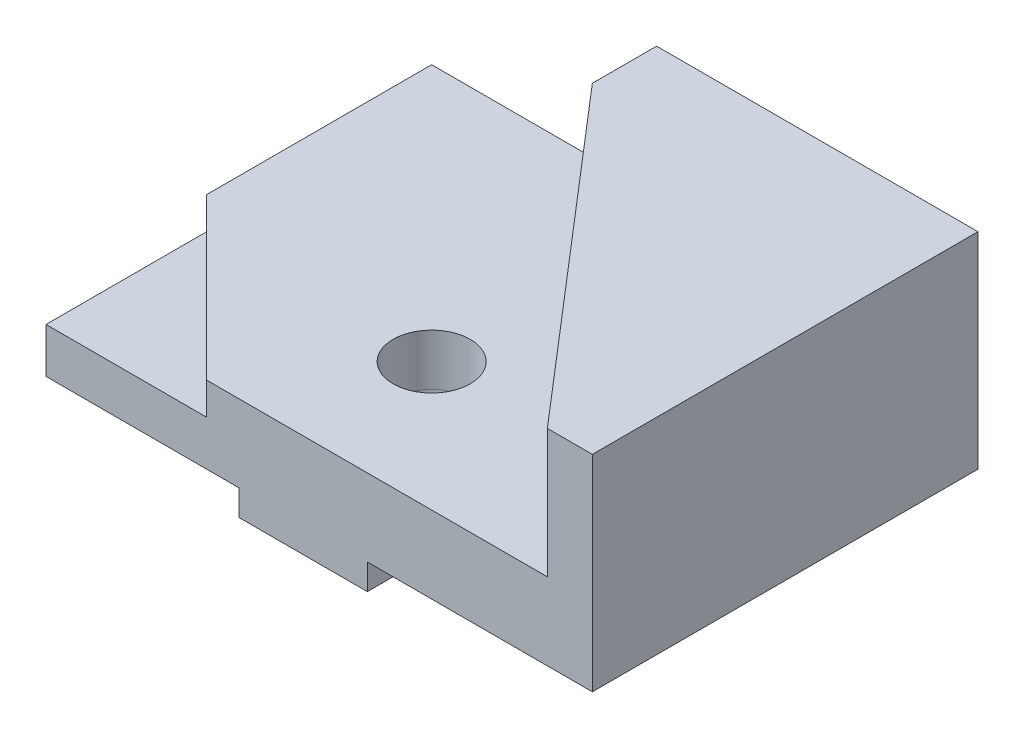
ISO-10303-21;
HEADER;
FILE_DESCRIPTION(('STEP AP214'),'2;1');
FILE_NAME('part.step','',(''),(''),'','','');
FILE_SCHEMA(('AUTOMOTIVE_DESIGN { 1 0 10303 214 1 1 1 1 }'));
ENDSEC;
DATA;
#1=APPLICATION_CONTEXT('core data for automotive mechanical design processes');
#2=APPLICATION_PROTOCOL_DEFINITION('international standard','automotive_design',2000,#1);
#3=PRODUCT_CONTEXT('',#1,'mechanical');
#4=PRODUCT('Part','Part','',(#3));
#5=PRODUCT_RELATED_PRODUCT_CATEGORY('part','',(#4));
#6=PRODUCT_DEFINITION_FORMATION('','',#4);
#7=PRODUCT_DEFINITION_CONTEXT('part definition',#1,'design');
#8=PRODUCT_DEFINITION('design','',#6,#7);
#9=PRODUCT_DEFINITION_SHAPE('','',#8);
#10=(LENGTH_UNIT() NAMED_UNIT(*) SI_UNIT(.MILLI.,.METRE.));
#11=(NAMED_UNIT(*) PLANE_ANGLE_UNIT() SI_UNIT($,.RADIAN.));
#12=(NAMED_UNIT(*) SI_UNIT($,.STERADIAN.) SOLID_ANGLE_UNIT());
#13=UNCERTAINTY_MEASURE_WITH_UNIT(LENGTH_MEASURE(1.E-05),#10,'distance_accuracy_value','');
#14=(GEOMETRIC_REPRESENTATION_CONTEXT(3) GLOBAL_UNCERTAINTY_ASSIGNED_CONTEXT((#13)) GLOBAL_UNIT_ASSIGNED_CONTEXT((#10,
#11,#12)) REPRESENTATION_CONTEXT('',''));
#15=CARTESIAN_POINT('',(0.,0.,0.));
#16=DIRECTION('',(0.,0.,1.));
#17=DIRECTION('',(1.,0.,0.));
#18=AXIS2_PLACEMENT_3D('',#15,#16,#17);
#19=CARTESIAN_POINT('',(0.,16.,0.));
#20=DIRECTION('',(0.,-1.,0.));
#21=DIRECTION('',(0.,0.,-1.));
#22=AXIS2_PLACEMENT_3D('',#19,#20,#21);
#23=PLANE('',#22);
#24=CARTESIAN_POINT('',(-10.,16.,-20.));
#25=DIRECTION('',(0.,1.,0.));
#26=DIRECTION('',(0.,0.,1.));
#27=AXIS2_PLACEMENT_3D('',#24,#25,#26);
#28=CIRCLE('',#27,6.);
#29=CARTESIAN_POINT('',(-10.,16.,-14.));
#30=VERTEX_POINT('',#29);
#31=EDGE_CURVE('E373',#30,#30,#28,.T.);
#32=ORIENTED_EDGE('',*,*,#31,.F.);
#33=EDGE_LOOP('',(#32));
#34=FACE_BOUND('',#33,.T.);
#35=DIRECTION('',(0.,0.,1.));
#36=VECTOR('',#35,1.);
#37=CARTESIAN_POINT('',(-50.,16.,0.));
#38=LINE('',#37,#36);
#39=CARTESIAN_POINT('',(-50.,16.,-60.));
#40=VERTEX_POINT('',#39);
#41=CARTESIAN_POINT('',(-50.,16.,-25.));
#42=VERTEX_POINT('',#41);
#43=EDGE_CURVE('E222',#40,#42,#38,.T.);
#44=ORIENTED_EDGE('',*,*,#43,.T.);
#45=DIRECTION('',(-0.707106781186547,0.,-0.707106781186547));
#46=VECTOR('',#45,1.);
#47=CARTESIAN_POINT('',(-25.,16.,0.));
#48=LINE('',#47,#46);
#49=CARTESIAN_POINT('',(-25.,16.,0.));
#50=VERTEX_POINT('',#49);
#51=EDGE_CURVE('E149',#50,#42,#48,.T.);
#52=ORIENTED_EDGE('',*,*,#51,.F.);
#53=DIRECTION('',(1.,0.,0.));
#54=VECTOR('',#53,1.);
#55=CARTESIAN_POINT('',(-50.,16.,0.));
#56=LINE('',#55,#54);
#57=CARTESIAN_POINT('',(28.,16.,0.));
#58=VERTEX_POINT('',#57);
#59=EDGE_CURVE('E152',#50,#58,#56,.T.);
#60=ORIENTED_EDGE('',*,*,#59,.T.);
#61=DIRECTION('',(0.652039268828047,0.,0.758185196311683));
#62=VECTOR('',#61,1.);
#63=CARTESIAN_POINT('',(-15.,16.,-50.));
#64=LINE('',#63,#62);
#65=CARTESIAN_POINT('',(-15.,16.,-50.));
#66=VERTEX_POINT('',#65);
#67=EDGE_CURVE('E161',#66,#58,#64,.T.);
#68=ORIENTED_EDGE('',*,*,#67,.F.);
#69=DIRECTION('',(0.,0.,1.));
#70=VECTOR('',#69,1.);
#71=CARTESIAN_POINT('',(-15.,16.,-60.));
#72=LINE('',#71,#70);
#73=CARTESIAN_POINT('',(-15.,16.,-60.));
#74=VERTEX_POINT('',#73);
#75=EDGE_CURVE('E61',#74,#66,#72,.T.);
#76=ORIENTED_EDGE('',*,*,#75,.F.);
#77=DIRECTION('',(-1.,0.,0.));
#78=VECTOR('',#77,1.);
#79=CARTESIAN_POINT('',(-50.,16.,-60.));
#80=LINE('',#79,#78);
#81=EDGE_CURVE('E228',#74,#40,#80,.T.);
#82=ORIENTED_EDGE('',*,*,#81,.T.);
#83=EDGE_LOOP('',(#44,#52,#60,#68,#76,#82));
#84=FACE_BOUND('',#83,.T.);
#85=ADVANCED_FACE('F41',(#34,#84),#23,.F.);
#86=CARTESIAN_POINT('',(-50.,16.,0.));
#87=DIRECTION('',(1.,0.,0.));
#88=DIRECTION('',(0.,0.,-1.));
#89=AXIS2_PLACEMENT_3D('',#86,#87,#88);
#90=PLANE('',#89);
#91=DIRECTION('',(0.,0.,1.));
#92=VECTOR('',#91,1.);
#93=CARTESIAN_POINT('',(-50.,11.,-25.));
#94=LINE('',#93,#92);
#95=CARTESIAN_POINT('',(-50.,11.,-25.));
#96=VERTEX_POINT('',#95);
#97=CARTESIAN_POINT('',(-50.,11.,0.));
#98=VERTEX_POINT('',#97);
#99=EDGE_CURVE('E57',#96,#98,#94,.T.);
#100=ORIENTED_EDGE('',*,*,#99,.F.);
#101=DIRECTION('',(0.,1.,0.));
#102=VECTOR('',#101,1.);
#103=CARTESIAN_POINT('',(-50.,11.,-25.));
#104=LINE('',#103,#102);
#105=EDGE_CURVE('E145',#96,#42,#104,.T.);
#106=ORIENTED_EDGE('',*,*,#105,.T.);
#107=ORIENTED_EDGE('',*,*,#43,.F.);
#108=DIRECTION('',(0.,-1.,0.));
#109=VECTOR('',#108,1.);
#110=CARTESIAN_POINT('',(-50.,16.,-60.));
#111=LINE('',#110,#109);
#112=CARTESIAN_POINT('',(-50.,4.,-60.));
#113=VERTEX_POINT('',#112);
#114=EDGE_CURVE('E226',#40,#113,#111,.T.);
#115=ORIENTED_EDGE('',*,*,#114,.T.);
#116=DIRECTION('',(0.,0.,1.));
#117=VECTOR('',#116,1.);
#118=CARTESIAN_POINT('',(-50.,4.,-60.));
#119=LINE('',#118,#117);
#120=CARTESIAN_POINT('',(-50.,4.,0.));
#121=VERTEX_POINT('',#120);
#122=EDGE_CURVE('E219',#113,#121,#119,.T.);
#123=ORIENTED_EDGE('',*,*,#122,.T.);
#124=DIRECTION('',(0.,-1.,0.));
#125=VECTOR('',#124,1.);
#126=CARTESIAN_POINT('',(-50.,16.,0.));
#127=LINE('',#126,#125);
#128=EDGE_CURVE('E239',#98,#121,#127,.T.);
#129=ORIENTED_EDGE('',*,*,#128,.F.);
#130=EDGE_LOOP('',(#100,#106,#107,#115,#123,#129));
#131=FACE_BOUND('',#130,.T.);
#132=ADVANCED_FACE('F253',(#131),#90,.F.);
#133=CARTESIAN_POINT('',(-50.,16.,0.));
#134=DIRECTION('',(0.,0.,-1.));
#135=DIRECTION('',(-1.,0.,0.));
#136=AXIS2_PLACEMENT_3D('',#133,#134,#135);
#137=PLANE('',#136);
#138=ORIENTED_EDGE('',*,*,#59,.F.);
#139=DIRECTION('',(0.,1.,0.));
#140=VECTOR('',#139,1.);
#141=CARTESIAN_POINT('',(-25.,11.,0.));
#142=LINE('',#141,#140);
#143=CARTESIAN_POINT('',(-25.,11.,0.));
#144=VERTEX_POINT('',#143);
#145=EDGE_CURVE('E136',#144,#50,#142,.T.);
#146=ORIENTED_EDGE('',*,*,#145,.F.);
#147=DIRECTION('',(1.,0.,0.));
#148=VECTOR('',#147,1.);
#149=CARTESIAN_POINT('',(-50.,11.,0.));
#150=LINE('',#149,#148);
#151=EDGE_CURVE('E141',#98,#144,#150,.T.);
#152=ORIENTED_EDGE('',*,*,#151,.F.);
#153=ORIENTED_EDGE('',*,*,#128,.T.);
#154=DIRECTION('',(-1.,0.,0.));
#155=VECTOR('',#154,1.);
#156=CARTESIAN_POINT('',(-20.,4.,0.));
#157=LINE('',#156,#155);
#158=CARTESIAN_POINT('',(-20.,4.,0.));
#159=VERTEX_POINT('',#158);
#160=EDGE_CURVE('E207',#159,#121,#157,.T.);
#161=ORIENTED_EDGE('',*,*,#160,.F.);
#162=DIRECTION('',(0.,1.,0.));
#163=VECTOR('',#162,1.);
#164=CARTESIAN_POINT('',(-20.,0.,0.));
#165=LINE('',#164,#163);
#166=CARTESIAN_POINT('',(-20.,0.,0.));
#167=VERTEX_POINT('',#166);
#168=EDGE_CURVE('E199',#167,#159,#165,.T.);
#169=ORIENTED_EDGE('',*,*,#168,.F.);
#170=DIRECTION('',(1.,0.,0.));
#171=VECTOR('',#170,1.);
#172=CARTESIAN_POINT('',(-50.,0.,0.));
#173=LINE('',#172,#171);
#174=CARTESIAN_POINT('',(0.,0.,0.));
#175=VERTEX_POINT('',#174);
#176=EDGE_CURVE('E218',#167,#175,#173,.T.);
#177=ORIENTED_EDGE('',*,*,#176,.T.);
#178=DIRECTION('',(0.,-1.,0.));
#179=VECTOR('',#178,1.);
#180=CARTESIAN_POINT('',(0.,4.,0.));
#181=LINE('',#180,#179);
#182=CARTESIAN_POINT('',(0.,4.,0.));
#183=VERTEX_POINT('',#182);
#184=EDGE_CURVE('E182',#183,#175,#181,.T.);
#185=ORIENTED_EDGE('',*,*,#184,.F.);
#186=DIRECTION('',(-1.,0.,0.));
#187=VECTOR('',#186,1.);
#188=CARTESIAN_POINT('',(35.,4.,0.));
#189=LINE('',#188,#187);
#190=CARTESIAN_POINT('',(35.,4.,0.));
#191=VERTEX_POINT('',#190);
#192=EDGE_CURVE('E189',#191,#183,#189,.T.);
#193=ORIENTED_EDGE('',*,*,#192,.F.);
#194=DIRECTION('',(0.,-1.,0.));
#195=VECTOR('',#194,1.);
#196=CARTESIAN_POINT('',(35.,16.,0.));
#197=LINE('',#196,#195);
#198=CARTESIAN_POINT('',(35.,36.,0.));
#199=VERTEX_POINT('',#198);
#200=EDGE_CURVE('E240',#199,#191,#197,.T.);
#201=ORIENTED_EDGE('',*,*,#200,.F.);
#202=DIRECTION('',(1.,0.,0.));
#203=VECTOR('',#202,1.);
#204=CARTESIAN_POINT('',(28.,36.,0.));
#205=LINE('',#204,#203);
#206=CARTESIAN_POINT('',(28.,36.,0.));
#207=VERTEX_POINT('',#206);
#208=EDGE_CURVE('E169',#207,#199,#205,.T.);
#209=ORIENTED_EDGE('',*,*,#208,.F.);
#210=DIRECTION('',(0.,-1.,0.));
#211=VECTOR('',#210,1.);
#212=CARTESIAN_POINT('',(28.,36.,0.));
#213=LINE('',#212,#211);
#214=EDGE_CURVE('E175',#207,#58,#213,.T.);
#215=ORIENTED_EDGE('',*,*,#214,.T.);
#216=EDGE_LOOP('',(#138,#146,#152,#153,#161,#169,#177,#185,#193,#201,#209,#215));
#217=FACE_BOUND('',#216,.T.);
#218=ADVANCED_FACE('F153',(#217),#137,.F.);
#219=CARTESIAN_POINT('',(35.,16.,0.));
#220=DIRECTION('',(-1.,0.,0.));
#221=DIRECTION('',(0.,0.,1.));
#222=AXIS2_PLACEMENT_3D('',#219,#220,#221);
#223=PLANE('',#222);
#224=ORIENTED_EDGE('',*,*,#200,.T.);
#225=DIRECTION('',(0.,0.,1.));
#226=VECTOR('',#225,1.);
#227=CARTESIAN_POINT('',(35.,4.,-60.));
#228=LINE('',#227,#226);
#229=CARTESIAN_POINT('',(35.,4.,-60.));
#230=VERTEX_POINT('',#229);
#231=EDGE_CURVE('E197',#230,#191,#228,.T.);
#232=ORIENTED_EDGE('',*,*,#231,.F.);
#233=DIRECTION('',(0.,-1.,0.));
#234=VECTOR('',#233,1.);
#235=CARTESIAN_POINT('',(35.,16.,-60.));
#236=LINE('',#235,#234);
#237=CARTESIAN_POINT('',(35.,36.,-60.));
#238=VERTEX_POINT('',#237);
#239=EDGE_CURVE('E234',#238,#230,#236,.T.);
#240=ORIENTED_EDGE('',*,*,#239,.F.);
#241=DIRECTION('',(0.,0.,-1.));
#242=VECTOR('',#241,1.);
#243=CARTESIAN_POINT('',(35.,36.,0.));
#244=LINE('',#243,#242);
#245=EDGE_CURVE('E156',#199,#238,#244,.T.);
#246=ORIENTED_EDGE('',*,*,#245,.F.);
#247=EDGE_LOOP('',(#224,#232,#240,#246));
#248=FACE_BOUND('',#247,.T.);
#249=ADVANCED_FACE('F277',(#248),#223,.F.);
#250=CARTESIAN_POINT('',(-50.,16.,-60.));
#251=DIRECTION('',(0.,0.,1.));
#252=DIRECTION('',(1.,0.,0.));
#253=AXIS2_PLACEMENT_3D('',#250,#251,#252);
#254=PLANE('',#253);
#255=DIRECTION('',(-1.,0.,0.));
#256=VECTOR('',#255,1.);
#257=CARTESIAN_POINT('',(35.,4.,-60.));
#258=LINE('',#257,#256);
#259=CARTESIAN_POINT('',(0.,4.,-60.));
#260=VERTEX_POINT('',#259);
#261=EDGE_CURVE('E190',#230,#260,#258,.T.);
#262=ORIENTED_EDGE('',*,*,#261,.T.);
#263=DIRECTION('',(0.,-1.,0.));
#264=VECTOR('',#263,1.);
#265=CARTESIAN_POINT('',(0.,4.,-60.));
#266=LINE('',#265,#264);
#267=CARTESIAN_POINT('',(0.,0.,-60.));
#268=VERTEX_POINT('',#267);
#269=EDGE_CURVE('E183',#260,#268,#266,.T.);
#270=ORIENTED_EDGE('',*,*,#269,.T.);
#271=DIRECTION('',(-1.,0.,0.));
#272=VECTOR('',#271,1.);
#273=CARTESIAN_POINT('',(-50.,0.,-60.));
#274=LINE('',#273,#272);
#275=CARTESIAN_POINT('',(-20.,0.,-60.));
#276=VERTEX_POINT('',#275);
#277=EDGE_CURVE('E221',#268,#276,#274,.T.);
#278=ORIENTED_EDGE('',*,*,#277,.T.);
#279=DIRECTION('',(0.,1.,0.));
#280=VECTOR('',#279,1.);
#281=CARTESIAN_POINT('',(-20.,0.,-60.));
#282=LINE('',#281,#280);
#283=CARTESIAN_POINT('',(-20.,4.,-60.));
#284=VERTEX_POINT('',#283);
#285=EDGE_CURVE('E205',#276,#284,#282,.T.);
#286=ORIENTED_EDGE('',*,*,#285,.T.);
#287=DIRECTION('',(-1.,0.,0.));
#288=VECTOR('',#287,1.);
#289=CARTESIAN_POINT('',(-20.,4.,-60.));
#290=LINE('',#289,#288);
#291=EDGE_CURVE('E203',#284,#113,#290,.T.);
#292=ORIENTED_EDGE('',*,*,#291,.T.);
#293=ORIENTED_EDGE('',*,*,#114,.F.);
#294=ORIENTED_EDGE('',*,*,#81,.F.);
#295=DIRECTION('',(0.,-1.,0.));
#296=VECTOR('',#295,1.);
#297=CARTESIAN_POINT('',(-15.,36.,-60.));
#298=LINE('',#297,#296);
#299=CARTESIAN_POINT('',(-15.,36.,-60.));
#300=VERTEX_POINT('',#299);
#301=EDGE_CURVE('E179',#300,#74,#298,.T.);
#302=ORIENTED_EDGE('',*,*,#301,.F.);
#303=DIRECTION('',(-1.,0.,0.));
#304=VECTOR('',#303,1.);
#305=CARTESIAN_POINT('',(35.,36.,-60.));
#306=LINE('',#305,#304);
#307=EDGE_CURVE('E162',#238,#300,#306,.T.);
#308=ORIENTED_EDGE('',*,*,#307,.F.);
#309=ORIENTED_EDGE('',*,*,#239,.T.);
#310=EDGE_LOOP('',(#262,#270,#278,#286,#292,#293,#294,#302,#308,#309));
#311=FACE_BOUND('',#310,.T.);
#312=ADVANCED_FACE('F275',(#311),#254,.F.);
#313=CARTESIAN_POINT('',(0.,0.,0.));
#314=DIRECTION('',(0.,-1.,0.));
#315=DIRECTION('',(0.,0.,-1.));
#316=AXIS2_PLACEMENT_3D('',#313,#314,#315);
#317=PLANE('',#316);
#318=DIRECTION('',(0.,0.,1.));
#319=VECTOR('',#318,1.);
#320=CARTESIAN_POINT('',(0.,0.,-60.));
#321=LINE('',#320,#319);
#322=EDGE_CURVE('E192',#268,#175,#321,.T.);
#323=ORIENTED_EDGE('',*,*,#322,.T.);
#324=ORIENTED_EDGE('',*,*,#176,.F.);
#325=DIRECTION('',(0.,0.,1.));
#326=VECTOR('',#325,1.);
#327=CARTESIAN_POINT('',(-20.,0.,-60.));
#328=LINE('',#327,#326);
#329=EDGE_CURVE('E211',#276,#167,#328,.T.);
#330=ORIENTED_EDGE('',*,*,#329,.F.);
#331=ORIENTED_EDGE('',*,*,#277,.F.);
#332=EDGE_LOOP('',(#323,#324,#330,#331));
#333=FACE_BOUND('',#332,.T.);
#334=ADVANCED_FACE('F266',(#333),#317,.T.);
#335=CARTESIAN_POINT('',(-20.,0.,-60.));
#336=DIRECTION('',(1.,0.,0.));
#337=DIRECTION('',(0.,0.,-1.));
#338=AXIS2_PLACEMENT_3D('',#335,#336,#337);
#339=PLANE('',#338);
#340=ORIENTED_EDGE('',*,*,#168,.T.);
#341=DIRECTION('',(0.,0.,1.));
#342=VECTOR('',#341,1.);
#343=CARTESIAN_POINT('',(-20.,4.,-60.));
#344=LINE('',#343,#342);
#345=EDGE_CURVE('E209',#284,#159,#344,.T.);
#346=ORIENTED_EDGE('',*,*,#345,.F.);
#347=ORIENTED_EDGE('',*,*,#285,.F.);
#348=ORIENTED_EDGE('',*,*,#329,.T.);
#349=EDGE_LOOP('',(#340,#346,#347,#348));
#350=FACE_BOUND('',#349,.T.);
#351=ADVANCED_FACE('F270',(#350),#339,.F.);
#352=CARTESIAN_POINT('',(-20.,4.,-60.));
#353=DIRECTION('',(0.,1.,0.));
#354=DIRECTION('',(-1.,0.,0.));
#355=AXIS2_PLACEMENT_3D('',#352,#353,#354);
#356=PLANE('',#355);
#357=ORIENTED_EDGE('',*,*,#160,.T.);
#358=ORIENTED_EDGE('',*,*,#122,.F.);
#359=ORIENTED_EDGE('',*,*,#291,.F.);
#360=ORIENTED_EDGE('',*,*,#345,.T.);
#361=EDGE_LOOP('',(#357,#358,#359,#360));
#362=FACE_BOUND('',#361,.T.);
#363=ADVANCED_FACE('F341',(#362),#356,.F.);
#364=CARTESIAN_POINT('',(0.,4.,-60.));
#365=DIRECTION('',(-1.,0.,0.));
#366=DIRECTION('',(0.,0.,1.));
#367=AXIS2_PLACEMENT_3D('',#364,#365,#366);
#368=PLANE('',#367);
#369=ORIENTED_EDGE('',*,*,#184,.T.);
#370=ORIENTED_EDGE('',*,*,#322,.F.);
#371=ORIENTED_EDGE('',*,*,#269,.F.);
#372=DIRECTION('',(0.,0.,1.));
#373=VECTOR('',#372,1.);
#374=CARTESIAN_POINT('',(0.,4.,-60.));
#375=LINE('',#374,#373);
#376=EDGE_CURVE('E193',#260,#183,#375,.T.);
#377=ORIENTED_EDGE('',*,*,#376,.T.);
#378=EDGE_LOOP('',(#369,#370,#371,#377));
#379=FACE_BOUND('',#378,.T.);
#380=ADVANCED_FACE('F342',(#379),#368,.F.);
#381=CARTESIAN_POINT('',(35.,4.,-60.));
#382=DIRECTION('',(0.,1.,0.));
#383=DIRECTION('',(-1.,0.,0.));
#384=AXIS2_PLACEMENT_3D('',#381,#382,#383);
#385=PLANE('',#384);
#386=ORIENTED_EDGE('',*,*,#192,.T.);
#387=ORIENTED_EDGE('',*,*,#376,.F.);
#388=ORIENTED_EDGE('',*,*,#261,.F.);
#389=ORIENTED_EDGE('',*,*,#231,.T.);
#390=EDGE_LOOP('',(#386,#387,#388,#389));
#391=FACE_BOUND('',#390,.T.);
#392=ADVANCED_FACE('F340',(#391),#385,.F.);
#393=CARTESIAN_POINT('',(-15.,36.,-60.));
#394=DIRECTION('',(1.,0.,0.));
#395=DIRECTION('',(0.,0.,-1.));
#396=AXIS2_PLACEMENT_3D('',#393,#394,#395);
#397=PLANE('',#396);
#398=ORIENTED_EDGE('',*,*,#75,.T.);
#399=DIRECTION('',(0.,-1.,0.));
#400=VECTOR('',#399,1.);
#401=CARTESIAN_POINT('',(-15.,36.,-50.));
#402=LINE('',#401,#400);
#403=CARTESIAN_POINT('',(-15.,36.,-50.));
#404=VERTEX_POINT('',#403);
#405=EDGE_CURVE('E180',#404,#66,#402,.T.);
#406=ORIENTED_EDGE('',*,*,#405,.F.);
#407=DIRECTION('',(0.,0.,1.));
#408=VECTOR('',#407,1.);
#409=CARTESIAN_POINT('',(-15.,36.,-60.));
#410=LINE('',#409,#408);
#411=EDGE_CURVE('E164',#300,#404,#410,.T.);
#412=ORIENTED_EDGE('',*,*,#411,.F.);
#413=ORIENTED_EDGE('',*,*,#301,.T.);
#414=EDGE_LOOP('',(#398,#406,#412,#413));
#415=FACE_BOUND('',#414,.T.);
#416=ADVANCED_FACE('F334',(#415),#397,.F.);
#417=CARTESIAN_POINT('',(-15.,36.,-50.));
#418=DIRECTION('',(0.758185196311683,0.,-0.652039268828047));
#419=DIRECTION('',(-0.652039268828047,0.,-0.758185196311683));
#420=AXIS2_PLACEMENT_3D('',#417,#418,#419);
#421=PLANE('',#420);
#422=ORIENTED_EDGE('',*,*,#67,.T.);
#423=ORIENTED_EDGE('',*,*,#214,.F.);
#424=DIRECTION('',(0.652039268828047,0.,0.758185196311683));
#425=VECTOR('',#424,1.);
#426=CARTESIAN_POINT('',(-15.,36.,-50.));
#427=LINE('',#426,#425);
#428=EDGE_CURVE('E170',#404,#207,#427,.T.);
#429=ORIENTED_EDGE('',*,*,#428,.F.);
#430=ORIENTED_EDGE('',*,*,#405,.T.);
#431=EDGE_LOOP('',(#422,#423,#429,#430));
#432=FACE_BOUND('',#431,.T.);
#433=ADVANCED_FACE('F330',(#432),#421,.F.);
#434=CARTESIAN_POINT('',(0.,36.,0.));
#435=DIRECTION('',(0.,1.,0.));
#436=DIRECTION('',(0.,0.,1.));
#437=AXIS2_PLACEMENT_3D('',#434,#435,#436);
#438=PLANE('',#437);
#439=ORIENTED_EDGE('',*,*,#245,.T.);
#440=ORIENTED_EDGE('',*,*,#307,.T.);
#441=ORIENTED_EDGE('',*,*,#411,.T.);
#442=ORIENTED_EDGE('',*,*,#428,.T.);
#443=ORIENTED_EDGE('',*,*,#208,.T.);
#444=EDGE_LOOP('',(#439,#440,#441,#442,#443));
#445=FACE_BOUND('',#444,.T.);
#446=ADVANCED_FACE('F294',(#445),#438,.T.);
#447=CARTESIAN_POINT('',(-25.,11.,0.));
#448=DIRECTION('',(0.707106781186548,0.,-0.707106781186548));
#449=DIRECTION('',(-0.707106781186548,0.,-0.707106781186548));
#450=AXIS2_PLACEMENT_3D('',#447,#448,#449);
#451=PLANE('',#450);
#452=ORIENTED_EDGE('',*,*,#51,.T.);
#453=ORIENTED_EDGE('',*,*,#105,.F.);
#454=DIRECTION('',(-0.707106781186547,0.,-0.707106781186547));
#455=VECTOR('',#454,1.);
#456=CARTESIAN_POINT('',(-25.,11.,0.));
#457=LINE('',#456,#455);
#458=EDGE_CURVE('E137',#144,#96,#457,.T.);
#459=ORIENTED_EDGE('',*,*,#458,.F.);
#460=ORIENTED_EDGE('',*,*,#145,.T.);
#461=EDGE_LOOP('',(#452,#453,#459,#460));
#462=FACE_BOUND('',#461,.T.);
#463=ADVANCED_FACE('F140',(#462),#451,.F.);
#464=CARTESIAN_POINT('',(0.,11.,0.));
#465=DIRECTION('',(0.,-1.,0.));
#466=DIRECTION('',(0.,0.,-1.));
#467=AXIS2_PLACEMENT_3D('',#464,#465,#466);
#468=PLANE('',#467);
#469=ORIENTED_EDGE('',*,*,#151,.T.);
#470=ORIENTED_EDGE('',*,*,#458,.T.);
#471=ORIENTED_EDGE('',*,*,#99,.T.);
#472=EDGE_LOOP('',(#469,#470,#471));
#473=FACE_BOUND('',#472,.T.);
#474=ADVANCED_FACE('F143',(#473),#468,.F.);
#475=CARTESIAN_POINT('',(-10.,6.,-20.));
#476=DIRECTION('',(0.,1.,0.));
#477=DIRECTION('',(0.,0.,1.));
#478=AXIS2_PLACEMENT_3D('',#475,#476,#477);
#479=CYLINDRICAL_SURFACE('',#478,6.);
#480=CARTESIAN_POINT('',(-10.,8.,-20.));
#481=DIRECTION('',(0.,1.,0.));
#482=DIRECTION('',(0.,0.,1.));
#483=AXIS2_PLACEMENT_3D('',#480,#481,#482);
#484=CIRCLE('',#483,6.);
#485=CARTESIAN_POINT('',(-10.,8.,-14.));
#486=VERTEX_POINT('',#485);
#487=EDGE_CURVE('E11',#486,#486,#484,.F.);
#488=ORIENTED_EDGE('',*,*,#487,.T.);
#489=EDGE_LOOP('',(#488));
#490=FACE_BOUND('',#489,.T.);
#491=ORIENTED_EDGE('',*,*,#31,.T.);
#492=EDGE_LOOP('',(#491));
#493=FACE_BOUND('',#492,.T.);
#494=ADVANCED_FACE('F252',(#490,#493),#479,.F.);
#495=CARTESIAN_POINT('',(-10.,6.,-20.));
#496=DIRECTION('',(0.,1.,0.));
#497=DIRECTION('',(0.,0.,1.));
#498=AXIS2_PLACEMENT_3D('',#495,#496,#497);
#499=PLANE('',#498);
#500=CARTESIAN_POINT('',(-10.,6.,-20.));
#501=DIRECTION('',(0.,1.,0.));
#502=DIRECTION('',(0.,0.,1.));
#503=AXIS2_PLACEMENT_3D('',#500,#501,#502);
#504=CIRCLE('',#503,4.);
#505=CARTESIAN_POINT('',(-10.,6.,-16.));
#506=VERTEX_POINT('',#505);
#507=EDGE_CURVE('E47',#506,#506,#504,.T.);
#508=ORIENTED_EDGE('',*,*,#507,.T.);
#509=EDGE_LOOP('',(#508));
#510=FACE_BOUND('',#509,.T.);
#511=ADVANCED_FACE('F242',(#510),#499,.T.);
#512=CARTESIAN_POINT('',(-10.,8.,-20.));
#513=DIRECTION('',(0.,1.,0.));
#514=DIRECTION('',(0.,0.,1.));
#515=AXIS2_PLACEMENT_3D('',#512,#513,#514);
#516=TOROIDAL_SURFACE('',#515,4.,2.);
#517=ORIENTED_EDGE('',*,*,#487,.F.);
#518=EDGE_LOOP('',(#517));
#519=FACE_BOUND('',#518,.T.);
#520=ORIENTED_EDGE('',*,*,#507,.F.);
#521=EDGE_LOOP('',(#520));
#522=FACE_BOUND('',#521,.T.);
#523=ADVANCED_FACE('F43',(#519,#522),#516,.F.);
#524=CLOSED_SHELL('',(#85,#132,#218,#249,#312,#334,#351,#363,#380,#392,#416,#433,#446,#463,#474,
#494,#511,#523));
#525=MANIFOLD_SOLID_BREP('B2',#524);
#526=ADVANCED_BREP_SHAPE_REPRESENTATION('',(#18,#525),#14);
#527=SHAPE_DEFINITION_REPRESENTATION(#9,#526);
ENDSEC;
END-ISO-10303-21;
